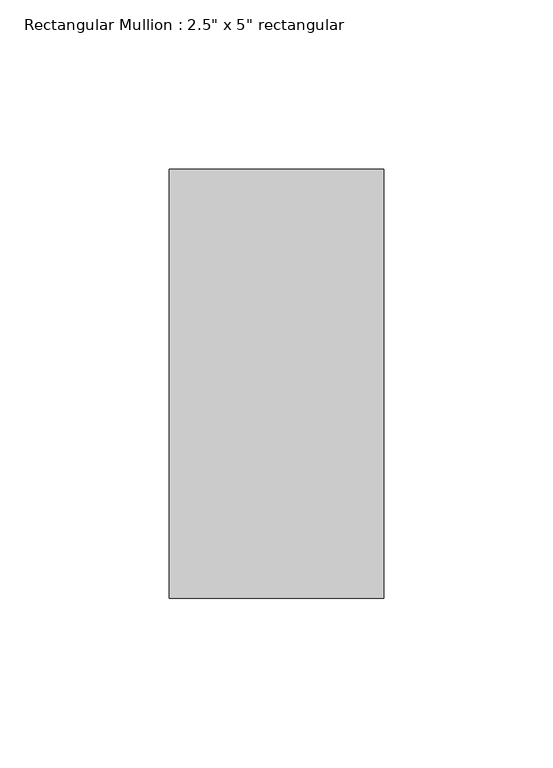
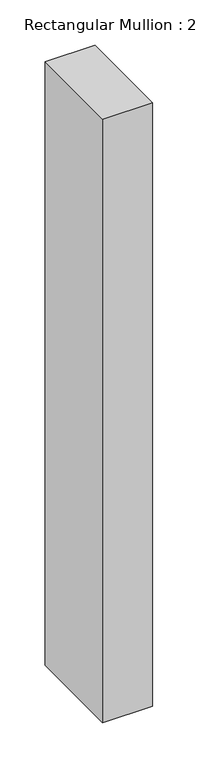
"""IFC4 building model written with IfcOpenShell, lengths in millimetres: member geometry."""

from ifc_helpers import new_model, si_unit, frame, origin, place, context, project, spatial, polyline, outline, extrude, source, transform, mapped, element, save


def member_8b3492ed(model_context):
    return source(origin(), model_context, "Body", "SweptSolid", [
        extrude(outline(polyline([(0.0, 63.5), (0.0, -63.5), (-63.5, -63.5), (-63.5, 63.5), (0.0, 63.5)])), frame((0.0, 0.0, -812.8), z_axis=(0.0, 0.0, 1.0), x_axis=(1.0, 0.0, 0.0)), (0.0, 0.0, 1.0), 812.8),
    ])


if __name__ == "__main__":
    model = new_model("IFC4")
    model_context = context("Model", 3, world=origin())
    ifc_project = project(units=[si_unit("LENGTHUNIT", "METRE", prefix="MILLI")], contexts=[model_context])
    site = spatial("IfcSite", under=ifc_project)
    building = spatial("IfcBuilding", under=site)
    placement = place(None, origin())
    member_shape = member_8b3492ed(model_context)
    element("IfcMember", 1, ObjectType="Rectangular Mullion : 2.5\" x 5\" rectangular", at=placement, inside=building, context=model_context, shape_type="MappedRepresentation", body=[
        mapped(member_shape, transform((0.0, 0.0, 0.0), x_axis=(1.0, 0.0, 0.0), y_axis=(0.0, 1.0, 0.0), z_axis=(0.0, 0.0, 1.0))),
    ])
    save(model, "model.ifc")

# Revit data of these elements
# Type "Rectangular Mullion : 2.5\" x 5\" rectangular"
#   built-in parameter 1007304 = 0.416667 (stored number, unit not read)
#   built-in parameter 1007301 = 0.104167 (stored number, unit not read)
#   built-in parameter 1007300 = 0.104167 (stored number, unit not read)
# Element 1 (IfcMember, "Rectangular Mullion : 2.5\" x 5\" rectangular")
#   Materials on its faces: "Aluminum"
# Materials
#   "Aluminum": class "Metal", colour RGB 247 247 247, transparency 0, Description = "Aluminum 6061", Cost = 0
